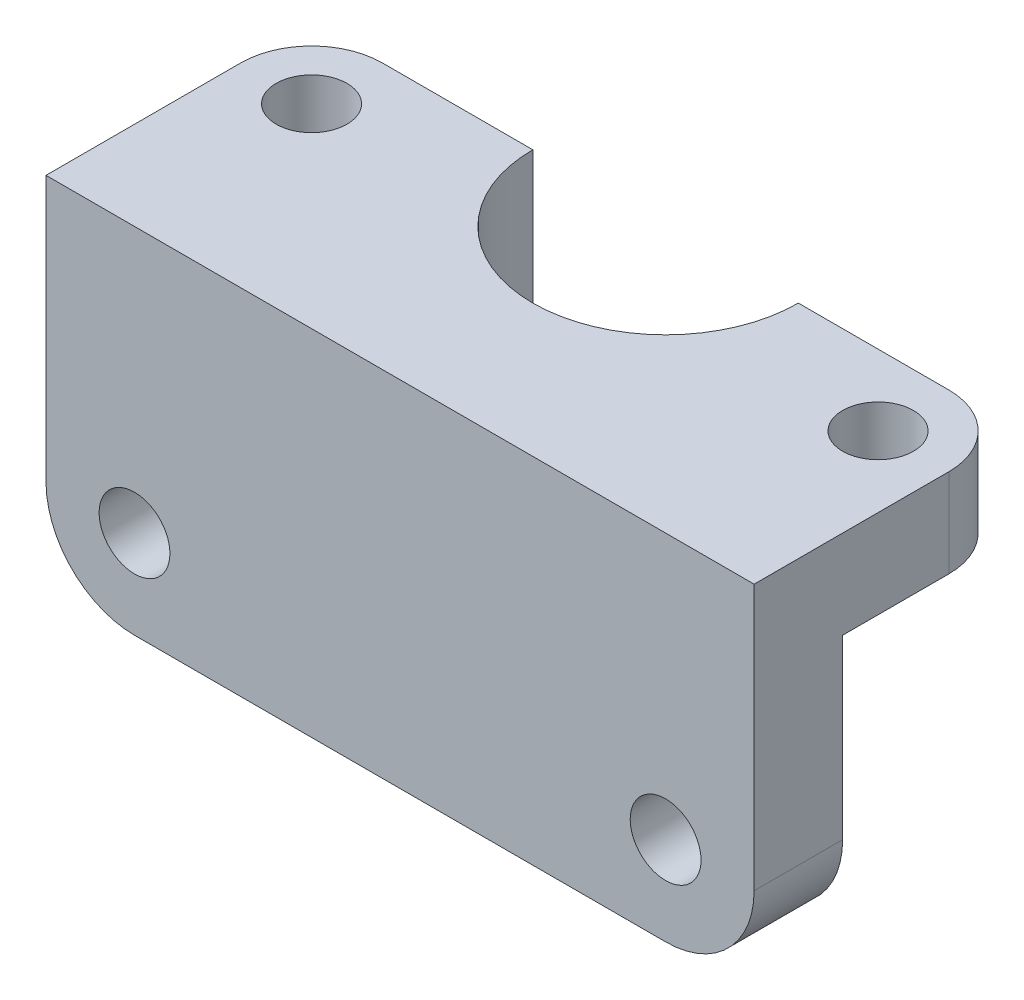
ISO-10303-21;
HEADER;
FILE_DESCRIPTION(('STEP AP214'),'2;1');
FILE_NAME('part.step','',(''),(''),'','','');
FILE_SCHEMA(('AUTOMOTIVE_DESIGN { 1 0 10303 214 1 1 1 1 }'));
ENDSEC;
DATA;
#1=APPLICATION_CONTEXT('core data for automotive mechanical design processes');
#2=APPLICATION_PROTOCOL_DEFINITION('international standard','automotive_design',2000,#1);
#3=PRODUCT_CONTEXT('',#1,'mechanical');
#4=PRODUCT('Part','Part','',(#3));
#5=PRODUCT_RELATED_PRODUCT_CATEGORY('part','',(#4));
#6=PRODUCT_DEFINITION_FORMATION('','',#4);
#7=PRODUCT_DEFINITION_CONTEXT('part definition',#1,'design');
#8=PRODUCT_DEFINITION('design','',#6,#7);
#9=PRODUCT_DEFINITION_SHAPE('','',#8);
#10=(LENGTH_UNIT() NAMED_UNIT(*) SI_UNIT(.MILLI.,.METRE.));
#11=(NAMED_UNIT(*) PLANE_ANGLE_UNIT() SI_UNIT($,.RADIAN.));
#12=(NAMED_UNIT(*) SI_UNIT($,.STERADIAN.) SOLID_ANGLE_UNIT());
#13=UNCERTAINTY_MEASURE_WITH_UNIT(LENGTH_MEASURE(1.E-05),#10,'distance_accuracy_value','');
#14=(GEOMETRIC_REPRESENTATION_CONTEXT(3) GLOBAL_UNCERTAINTY_ASSIGNED_CONTEXT((#13)) GLOBAL_UNIT_ASSIGNED_CONTEXT((#10,
#11,#12)) REPRESENTATION_CONTEXT('',''));
#15=CARTESIAN_POINT('',(0.,0.,0.));
#16=DIRECTION('',(0.,0.,1.));
#17=DIRECTION('',(1.,0.,0.));
#18=AXIS2_PLACEMENT_3D('',#15,#16,#17);
#19=CARTESIAN_POINT('',(8.00000000000006,-10.,-20.));
#20=DIRECTION('',(0.,0.,-1.));
#21=DIRECTION('',(-1.,0.,0.));
#22=AXIS2_PLACEMENT_3D('',#19,#20,#21);
#23=PLANE('',#22);
#24=DIRECTION('',(0.,-1.,0.));
#25=VECTOR('',#24,1.);
#26=CARTESIAN_POINT('',(55.,0.,-20.));
#27=LINE('',#26,#25);
#28=CARTESIAN_POINT('',(55.,0.,-20.));
#29=VERTEX_POINT('',#28);
#30=CARTESIAN_POINT('',(55.,-35.,-20.));
#31=VERTEX_POINT('',#30);
#32=EDGE_CURVE('E62',#29,#31,#27,.T.);
#33=ORIENTED_EDGE('',*,*,#32,.F.);
#34=DIRECTION('',(-1.,0.,0.));
#35=VECTOR('',#34,1.);
#36=CARTESIAN_POINT('',(8.00000000000006,0.,-20.));
#37=LINE('',#36,#35);
#38=CARTESIAN_POINT('',(71.9999999999999,0.,-20.));
#39=VERTEX_POINT('',#38);
#40=EDGE_CURVE('E179',#39,#29,#37,.T.);
#41=ORIENTED_EDGE('',*,*,#40,.F.);
#42=DIRECTION('',(0.,1.,0.));
#43=VECTOR('',#42,1.);
#44=CARTESIAN_POINT('',(71.9999999999999,-10.,-20.));
#45=LINE('',#44,#43);
#46=CARTESIAN_POINT('',(71.9999999999999,-10.,-20.));
#47=VERTEX_POINT('',#46);
#48=EDGE_CURVE('E199',#47,#39,#45,.T.);
#49=ORIENTED_EDGE('',*,*,#48,.F.);
#50=DIRECTION('',(-1.,0.,0.));
#51=VECTOR('',#50,1.);
#52=CARTESIAN_POINT('',(8.00000000000006,-10.,-20.));
#53=LINE('',#52,#51);
#54=CARTESIAN_POINT('',(60.,-10.,-20.));
#55=VERTEX_POINT('',#54);
#56=EDGE_CURVE('E295',#47,#55,#53,.T.);
#57=ORIENTED_EDGE('',*,*,#56,.T.);
#58=DIRECTION('',(0.,1.,0.));
#59=VECTOR('',#58,1.);
#60=CARTESIAN_POINT('',(60.,-35.,-20.));
#61=LINE('',#60,#59);
#62=CARTESIAN_POINT('',(60.,-35.,-20.));
#63=VERTEX_POINT('',#62);
#64=EDGE_CURVE('E281',#63,#55,#61,.T.);
#65=ORIENTED_EDGE('',*,*,#64,.F.);
#66=DIRECTION('',(1.,0.,0.));
#67=VECTOR('',#66,1.);
#68=CARTESIAN_POINT('',(20.,-35.,-20.));
#69=LINE('',#68,#67);
#70=EDGE_CURVE('E269',#31,#63,#69,.T.);
#71=ORIENTED_EDGE('',*,*,#70,.F.);
#72=EDGE_LOOP('',(#33,#41,#49,#57,#65,#71));
#73=FACE_BOUND('',#72,.T.);
#74=ADVANCED_FACE('F44',(#73),#23,.T.);
#75=CARTESIAN_POINT('',(70.,-30.,0.));
#76=DIRECTION('',(0.,0.,1.));
#77=DIRECTION('',(1.,0.,0.));
#78=AXIS2_PLACEMENT_3D('',#75,#76,#77);
#79=PLANE('',#78);
#80=CARTESIAN_POINT('',(70.,-30.,0.));
#81=DIRECTION('',(0.,0.,-1.));
#82=DIRECTION('',(-1.,0.,0.));
#83=AXIS2_PLACEMENT_3D('',#80,#81,#82);
#84=CIRCLE('',#83,4.00000000000001);
#85=CARTESIAN_POINT('',(66.,-30.,0.));
#86=VERTEX_POINT('',#85);
#87=EDGE_CURVE('E242',#86,#86,#84,.T.);
#88=ORIENTED_EDGE('',*,*,#87,.F.);
#89=EDGE_LOOP('',(#88));
#90=FACE_BOUND('',#89,.T.);
#91=CARTESIAN_POINT('',(10.,-30.,0.));
#92=DIRECTION('',(0.,0.,-1.));
#93=DIRECTION('',(-1.,0.,0.));
#94=AXIS2_PLACEMENT_3D('',#91,#92,#93);
#95=CIRCLE('',#94,4.);
#96=CARTESIAN_POINT('',(6.,-30.,0.));
#97=VERTEX_POINT('',#96);
#98=EDGE_CURVE('E246',#97,#97,#95,.T.);
#99=ORIENTED_EDGE('',*,*,#98,.F.);
#100=EDGE_LOOP('',(#99));
#101=FACE_BOUND('',#100,.T.);
#102=DIRECTION('',(0.,1.,0.));
#103=VECTOR('',#102,1.);
#104=CARTESIAN_POINT('',(20.,-35.,0.));
#105=LINE('',#104,#103);
#106=CARTESIAN_POINT('',(20.,-35.,0.));
#107=VERTEX_POINT('',#106);
#108=CARTESIAN_POINT('',(20.,-10.,0.));
#109=VERTEX_POINT('',#108);
#110=EDGE_CURVE('E186',#107,#109,#105,.T.);
#111=ORIENTED_EDGE('',*,*,#110,.F.);
#112=DIRECTION('',(-1.,0.,0.));
#113=VECTOR('',#112,1.);
#114=CARTESIAN_POINT('',(40.,-35.,0.));
#115=LINE('',#114,#113);
#116=CARTESIAN_POINT('',(60.,-35.,0.));
#117=VERTEX_POINT('',#116);
#118=EDGE_CURVE('E66',#117,#107,#115,.T.);
#119=ORIENTED_EDGE('',*,*,#118,.F.);
#120=DIRECTION('',(0.,1.,0.));
#121=VECTOR('',#120,1.);
#122=CARTESIAN_POINT('',(60.,-35.,0.));
#123=LINE('',#122,#121);
#124=CARTESIAN_POINT('',(60.,-10.,0.));
#125=VERTEX_POINT('',#124);
#126=EDGE_CURVE('E274',#117,#125,#123,.T.);
#127=ORIENTED_EDGE('',*,*,#126,.T.);
#128=DIRECTION('',(1.,0.,0.));
#129=VECTOR('',#128,1.);
#130=CARTESIAN_POINT('',(80.,-10.,0.));
#131=LINE('',#130,#129);
#132=CARTESIAN_POINT('',(80.,-10.,0.));
#133=VERTEX_POINT('',#132);
#134=EDGE_CURVE('E303',#125,#133,#131,.T.);
#135=ORIENTED_EDGE('',*,*,#134,.T.);
#136=DIRECTION('',(0.,1.,0.));
#137=VECTOR('',#136,1.);
#138=CARTESIAN_POINT('',(80.,0.,0.));
#139=LINE('',#138,#137);
#140=CARTESIAN_POINT('',(80.,-29.9999999999999,0.));
#141=VERTEX_POINT('',#140);
#142=EDGE_CURVE('E210',#141,#133,#139,.T.);
#143=ORIENTED_EDGE('',*,*,#142,.F.);
#144=CARTESIAN_POINT('',(70.,-30.,0.));
#145=DIRECTION('',(0.,0.,1.));
#146=DIRECTION('',(1.,0.,0.));
#147=AXIS2_PLACEMENT_3D('',#144,#145,#146);
#148=CIRCLE('',#147,10.);
#149=CARTESIAN_POINT('',(69.9999999999999,-40.,0.));
#150=VERTEX_POINT('',#149);
#151=EDGE_CURVE('E224',#150,#141,#148,.T.);
#152=ORIENTED_EDGE('',*,*,#151,.F.);
#153=DIRECTION('',(1.,0.,0.));
#154=VECTOR('',#153,1.);
#155=CARTESIAN_POINT('',(69.9999999999999,-40.,0.));
#156=LINE('',#155,#154);
#157=CARTESIAN_POINT('',(10.0000000000001,-40.,0.));
#158=VERTEX_POINT('',#157);
#159=EDGE_CURVE('E222',#158,#150,#156,.T.);
#160=ORIENTED_EDGE('',*,*,#159,.F.);
#161=CARTESIAN_POINT('',(10.,-30.,0.));
#162=DIRECTION('',(0.,0.,1.));
#163=DIRECTION('',(-1.,0.,0.));
#164=AXIS2_PLACEMENT_3D('',#161,#162,#163);
#165=CIRCLE('',#164,10.);
#166=CARTESIAN_POINT('',(0.,-30.,0.));
#167=VERTEX_POINT('',#166);
#168=EDGE_CURVE('E218',#167,#158,#165,.T.);
#169=ORIENTED_EDGE('',*,*,#168,.F.);
#170=DIRECTION('',(0.,-1.,0.));
#171=VECTOR('',#170,1.);
#172=CARTESIAN_POINT('',(0.,-29.9999999999999,0.));
#173=LINE('',#172,#171);
#174=CARTESIAN_POINT('',(0.,-10.,0.));
#175=VERTEX_POINT('',#174);
#176=EDGE_CURVE('E191',#175,#167,#173,.T.);
#177=ORIENTED_EDGE('',*,*,#176,.F.);
#178=EDGE_CURVE('E304',#175,#109,#131,.T.);
#179=ORIENTED_EDGE('',*,*,#178,.T.);
#180=EDGE_LOOP('',(#111,#119,#127,#135,#143,#152,#160,#169,#177,#179));
#181=FACE_BOUND('',#180,.T.);
#182=ADVANCED_FACE('F329',(#90,#101,#181),#79,.F.);
#183=CARTESIAN_POINT('',(72.,-10.,-12.));
#184=DIRECTION('',(0.,1.,0.));
#185=DIRECTION('',(0.,0.,1.));
#186=AXIS2_PLACEMENT_3D('',#183,#184,#185);
#187=PLANE('',#186);
#188=CARTESIAN_POINT('',(8.,-10.,-12.));
#189=DIRECTION('',(0.,-1.,0.));
#190=DIRECTION('',(0.,0.,-1.));
#191=AXIS2_PLACEMENT_3D('',#188,#189,#190);
#192=CIRCLE('',#191,4.);
#193=CARTESIAN_POINT('',(8.,-10.,-16.));
#194=VERTEX_POINT('',#193);
#195=EDGE_CURVE('E252',#194,#194,#192,.T.);
#196=ORIENTED_EDGE('',*,*,#195,.F.);
#197=EDGE_LOOP('',(#196));
#198=FACE_BOUND('',#197,.T.);
#199=DIRECTION('',(0.,0.,-1.));
#200=VECTOR('',#199,1.);
#201=CARTESIAN_POINT('',(20.,-10.,0.));
#202=LINE('',#201,#200);
#203=CARTESIAN_POINT('',(20.,-10.,-20.));
#204=VERTEX_POINT('',#203);
#205=EDGE_CURVE('E262',#109,#204,#202,.T.);
#206=ORIENTED_EDGE('',*,*,#205,.F.);
#207=ORIENTED_EDGE('',*,*,#178,.F.);
#208=DIRECTION('',(0.,0.,1.));
#209=VECTOR('',#208,1.);
#210=CARTESIAN_POINT('',(0.,-10.,0.));
#211=LINE('',#210,#209);
#212=CARTESIAN_POINT('',(0.,-10.,-11.9999999999999));
#213=VERTEX_POINT('',#212);
#214=EDGE_CURVE('E299',#213,#175,#211,.T.);
#215=ORIENTED_EDGE('',*,*,#214,.F.);
#216=CARTESIAN_POINT('',(8.,-10.,-12.));
#217=DIRECTION('',(0.,1.,0.));
#218=DIRECTION('',(0.,0.,1.));
#219=AXIS2_PLACEMENT_3D('',#216,#217,#218);
#220=CIRCLE('',#219,8.);
#221=CARTESIAN_POINT('',(8.00000000000006,-10.,-20.));
#222=VERTEX_POINT('',#221);
#223=EDGE_CURVE('E293',#222,#213,#220,.T.);
#224=ORIENTED_EDGE('',*,*,#223,.F.);
#225=EDGE_CURVE('E292',#204,#222,#53,.T.);
#226=ORIENTED_EDGE('',*,*,#225,.F.);
#227=EDGE_LOOP('',(#206,#207,#215,#224,#226));
#228=FACE_BOUND('',#227,.T.);
#229=ADVANCED_FACE('F347',(#198,#228),#187,.F.);
#230=CARTESIAN_POINT('',(72.,-10.,-12.));
#231=DIRECTION('',(0.,-1.,0.));
#232=DIRECTION('',(0.,0.,-1.));
#233=AXIS2_PLACEMENT_3D('',#230,#231,#232);
#234=CIRCLE('',#233,4.00000000000001);
#235=CARTESIAN_POINT('',(72.,-10.,-16.));
#236=VERTEX_POINT('',#235);
#237=EDGE_CURVE('E248',#236,#236,#234,.T.);
#238=ORIENTED_EDGE('',*,*,#237,.F.);
#239=EDGE_LOOP('',(#238));
#240=FACE_BOUND('',#239,.T.);
#241=DIRECTION('',(0.,0.,1.));
#242=VECTOR('',#241,1.);
#243=CARTESIAN_POINT('',(60.,-10.,-20.));
#244=LINE('',#243,#242);
#245=EDGE_CURVE('E268',#55,#125,#244,.T.);
#246=ORIENTED_EDGE('',*,*,#245,.F.);
#247=ORIENTED_EDGE('',*,*,#56,.F.);
#248=CARTESIAN_POINT('',(72.,-10.,-12.));
#249=DIRECTION('',(0.,1.,0.));
#250=DIRECTION('',(0.,0.,1.));
#251=AXIS2_PLACEMENT_3D('',#248,#249,#250);
#252=CIRCLE('',#251,8.);
#253=CARTESIAN_POINT('',(80.,-10.,-11.9999999999999));
#254=VERTEX_POINT('',#253);
#255=EDGE_CURVE('E193',#254,#47,#252,.T.);
#256=ORIENTED_EDGE('',*,*,#255,.F.);
#257=DIRECTION('',(0.,0.,-1.));
#258=VECTOR('',#257,1.);
#259=CARTESIAN_POINT('',(80.,-10.,-11.9999999999999));
#260=LINE('',#259,#258);
#261=EDGE_CURVE('E205',#133,#254,#260,.T.);
#262=ORIENTED_EDGE('',*,*,#261,.F.);
#263=ORIENTED_EDGE('',*,*,#134,.F.);
#264=EDGE_LOOP('',(#246,#247,#256,#262,#263));
#265=FACE_BOUND('',#264,.T.);
#266=ADVANCED_FACE('F311',(#240,#265),#187,.F.);
#267=CARTESIAN_POINT('',(0.,-29.9999999999999,10.));
#268=DIRECTION('',(1.,0.,0.));
#269=DIRECTION('',(0.,0.,-1.));
#270=AXIS2_PLACEMENT_3D('',#267,#268,#269);
#271=PLANE('',#270);
#272=DIRECTION('',(0.,0.,-1.));
#273=VECTOR('',#272,1.);
#274=CARTESIAN_POINT('',(0.,0.,10.));
#275=LINE('',#274,#273);
#276=CARTESIAN_POINT('',(0.,0.,10.));
#277=VERTEX_POINT('',#276);
#278=CARTESIAN_POINT('',(0.,0.,-11.9999999999999));
#279=VERTEX_POINT('',#278);
#280=EDGE_CURVE('E220',#277,#279,#275,.T.);
#281=ORIENTED_EDGE('',*,*,#280,.T.);
#282=DIRECTION('',(0.,1.,0.));
#283=VECTOR('',#282,1.);
#284=CARTESIAN_POINT('',(0.,-10.,-11.9999999999999));
#285=LINE('',#284,#283);
#286=EDGE_CURVE('E198',#213,#279,#285,.T.);
#287=ORIENTED_EDGE('',*,*,#286,.F.);
#288=ORIENTED_EDGE('',*,*,#214,.T.);
#289=ORIENTED_EDGE('',*,*,#176,.T.);
#290=DIRECTION('',(0.,0.,-1.));
#291=VECTOR('',#290,1.);
#292=CARTESIAN_POINT('',(0.,-30.,10.));
#293=LINE('',#292,#291);
#294=CARTESIAN_POINT('',(0.,-30.,10.));
#295=VERTEX_POINT('',#294);
#296=EDGE_CURVE('E11',#295,#167,#293,.T.);
#297=ORIENTED_EDGE('',*,*,#296,.F.);
#298=DIRECTION('',(0.,-1.,0.));
#299=VECTOR('',#298,1.);
#300=CARTESIAN_POINT('',(0.,-29.9999999999999,10.));
#301=LINE('',#300,#299);
#302=EDGE_CURVE('E201',#277,#295,#301,.T.);
#303=ORIENTED_EDGE('',*,*,#302,.F.);
#304=EDGE_LOOP('',(#281,#287,#288,#289,#297,#303));
#305=FACE_BOUND('',#304,.T.);
#306=ADVANCED_FACE('F50',(#305),#271,.F.);
#307=CARTESIAN_POINT('',(10.,-30.,10.));
#308=DIRECTION('',(0.,0.,-1.));
#309=DIRECTION('',(-1.,0.,0.));
#310=AXIS2_PLACEMENT_3D('',#307,#308,#309);
#311=CYLINDRICAL_SURFACE('',#310,10.);
#312=ORIENTED_EDGE('',*,*,#168,.T.);
#313=DIRECTION('',(0.,0.,-1.));
#314=VECTOR('',#313,1.);
#315=CARTESIAN_POINT('',(10.0000000000001,-40.,10.));
#316=LINE('',#315,#314);
#317=CARTESIAN_POINT('',(10.0000000000001,-40.,10.));
#318=VERTEX_POINT('',#317);
#319=EDGE_CURVE('E53',#318,#158,#316,.T.);
#320=ORIENTED_EDGE('',*,*,#319,.F.);
#321=CARTESIAN_POINT('',(10.,-30.,10.));
#322=DIRECTION('',(0.,0.,1.));
#323=DIRECTION('',(-1.,0.,0.));
#324=AXIS2_PLACEMENT_3D('',#321,#322,#323);
#325=CIRCLE('',#324,10.);
#326=EDGE_CURVE('E206',#295,#318,#325,.T.);
#327=ORIENTED_EDGE('',*,*,#326,.F.);
#328=ORIENTED_EDGE('',*,*,#296,.T.);
#329=EDGE_LOOP('',(#312,#320,#327,#328));
#330=FACE_BOUND('',#329,.T.);
#331=ADVANCED_FACE('F359',(#330),#311,.T.);
#332=CARTESIAN_POINT('',(69.9999999999999,-40.,10.));
#333=DIRECTION('',(0.,1.,0.));
#334=DIRECTION('',(0.,0.,1.));
#335=AXIS2_PLACEMENT_3D('',#332,#333,#334);
#336=PLANE('',#335);
#337=ORIENTED_EDGE('',*,*,#159,.T.);
#338=DIRECTION('',(0.,0.,-1.));
#339=VECTOR('',#338,1.);
#340=CARTESIAN_POINT('',(69.9999999999999,-40.,10.));
#341=LINE('',#340,#339);
#342=CARTESIAN_POINT('',(69.9999999999999,-40.,10.));
#343=VERTEX_POINT('',#342);
#344=EDGE_CURVE('E232',#343,#150,#341,.T.);
#345=ORIENTED_EDGE('',*,*,#344,.F.);
#346=DIRECTION('',(1.,0.,0.));
#347=VECTOR('',#346,1.);
#348=CARTESIAN_POINT('',(69.9999999999999,-40.,10.));
#349=LINE('',#348,#347);
#350=EDGE_CURVE('E207',#318,#343,#349,.T.);
#351=ORIENTED_EDGE('',*,*,#350,.F.);
#352=ORIENTED_EDGE('',*,*,#319,.T.);
#353=EDGE_LOOP('',(#337,#345,#351,#352));
#354=FACE_BOUND('',#353,.T.);
#355=ADVANCED_FACE('F360',(#354),#336,.F.);
#356=CARTESIAN_POINT('',(70.,-30.,10.));
#357=DIRECTION('',(0.,0.,-1.));
#358=DIRECTION('',(-1.,0.,0.));
#359=AXIS2_PLACEMENT_3D('',#356,#357,#358);
#360=CYLINDRICAL_SURFACE('',#359,10.);
#361=ORIENTED_EDGE('',*,*,#151,.T.);
#362=DIRECTION('',(0.,0.,-1.));
#363=VECTOR('',#362,1.);
#364=CARTESIAN_POINT('',(80.,-29.9999999999999,10.));
#365=LINE('',#364,#363);
#366=CARTESIAN_POINT('',(80.,-29.9999999999999,10.));
#367=VERTEX_POINT('',#366);
#368=EDGE_CURVE('E230',#367,#141,#365,.T.);
#369=ORIENTED_EDGE('',*,*,#368,.F.);
#370=CARTESIAN_POINT('',(70.,-30.,10.));
#371=DIRECTION('',(0.,0.,1.));
#372=DIRECTION('',(1.,0.,0.));
#373=AXIS2_PLACEMENT_3D('',#370,#371,#372);
#374=CIRCLE('',#373,10.);
#375=EDGE_CURVE('E211',#343,#367,#374,.T.);
#376=ORIENTED_EDGE('',*,*,#375,.F.);
#377=ORIENTED_EDGE('',*,*,#344,.T.);
#378=EDGE_LOOP('',(#361,#369,#376,#377));
#379=FACE_BOUND('',#378,.T.);
#380=ADVANCED_FACE('F330',(#379),#360,.T.);
#381=CARTESIAN_POINT('',(80.,0.,10.));
#382=DIRECTION('',(-1.,0.,0.));
#383=DIRECTION('',(0.,0.,1.));
#384=AXIS2_PLACEMENT_3D('',#381,#382,#383);
#385=PLANE('',#384);
#386=ORIENTED_EDGE('',*,*,#142,.T.);
#387=ORIENTED_EDGE('',*,*,#261,.T.);
#388=DIRECTION('',(0.,1.,0.));
#389=VECTOR('',#388,1.);
#390=CARTESIAN_POINT('',(80.,-10.,-11.9999999999999));
#391=LINE('',#390,#389);
#392=CARTESIAN_POINT('',(80.,0.,-11.9999999999999));
#393=VERTEX_POINT('',#392);
#394=EDGE_CURVE('E194',#254,#393,#391,.T.);
#395=ORIENTED_EDGE('',*,*,#394,.T.);
#396=DIRECTION('',(0.,0.,-1.));
#397=VECTOR('',#396,1.);
#398=CARTESIAN_POINT('',(80.,0.,10.));
#399=LINE('',#398,#397);
#400=CARTESIAN_POINT('',(80.,0.,10.));
#401=VERTEX_POINT('',#400);
#402=EDGE_CURVE('E229',#401,#393,#399,.T.);
#403=ORIENTED_EDGE('',*,*,#402,.F.);
#404=DIRECTION('',(0.,1.,0.));
#405=VECTOR('',#404,1.);
#406=CARTESIAN_POINT('',(80.,0.,10.));
#407=LINE('',#406,#405);
#408=EDGE_CURVE('E213',#367,#401,#407,.T.);
#409=ORIENTED_EDGE('',*,*,#408,.F.);
#410=ORIENTED_EDGE('',*,*,#368,.T.);
#411=EDGE_LOOP('',(#386,#387,#395,#403,#409,#410));
#412=FACE_BOUND('',#411,.T.);
#413=ADVANCED_FACE('F307',(#412),#385,.F.);
#414=CARTESIAN_POINT('',(0.,0.,10.));
#415=DIRECTION('',(0.,-1.,0.));
#416=DIRECTION('',(0.,0.,-1.));
#417=AXIS2_PLACEMENT_3D('',#414,#415,#416);
#418=PLANE('',#417);
#419=CARTESIAN_POINT('',(72.,0.,-12.));
#420=DIRECTION('',(0.,-1.,0.));
#421=DIRECTION('',(0.,0.,-1.));
#422=AXIS2_PLACEMENT_3D('',#419,#420,#421);
#423=CIRCLE('',#422,4.00000000000001);
#424=CARTESIAN_POINT('',(72.,0.,-16.));
#425=VERTEX_POINT('',#424);
#426=EDGE_CURVE('E47',#425,#425,#423,.T.);
#427=ORIENTED_EDGE('',*,*,#426,.T.);
#428=EDGE_LOOP('',(#427));
#429=FACE_BOUND('',#428,.T.);
#430=CARTESIAN_POINT('',(8.,0.,-12.));
#431=DIRECTION('',(0.,-1.,0.));
#432=DIRECTION('',(0.,0.,-1.));
#433=AXIS2_PLACEMENT_3D('',#430,#431,#432);
#434=CIRCLE('',#433,4.);
#435=CARTESIAN_POINT('',(8.,0.,-16.));
#436=VERTEX_POINT('',#435);
#437=EDGE_CURVE('E243',#436,#436,#434,.T.);
#438=ORIENTED_EDGE('',*,*,#437,.T.);
#439=EDGE_LOOP('',(#438));
#440=FACE_BOUND('',#439,.T.);
#441=ORIENTED_EDGE('',*,*,#40,.T.);
#442=CARTESIAN_POINT('',(40.,0.,-20.));
#443=DIRECTION('',(0.,-1.,0.));
#444=DIRECTION('',(0.,0.,-1.));
#445=AXIS2_PLACEMENT_3D('',#442,#443,#444);
#446=CIRCLE('',#445,15.);
#447=CARTESIAN_POINT('',(25.,0.,-20.));
#448=VERTEX_POINT('',#447);
#449=EDGE_CURVE('E165',#29,#448,#446,.T.);
#450=ORIENTED_EDGE('',*,*,#449,.T.);
#451=CARTESIAN_POINT('',(8.00000000000006,0.,-20.));
#452=VERTEX_POINT('',#451);
#453=EDGE_CURVE('E174',#448,#452,#37,.T.);
#454=ORIENTED_EDGE('',*,*,#453,.T.);
#455=CARTESIAN_POINT('',(8.,0.,-12.));
#456=DIRECTION('',(0.,1.,0.));
#457=DIRECTION('',(0.,0.,1.));
#458=AXIS2_PLACEMENT_3D('',#455,#456,#457);
#459=CIRCLE('',#458,8.);
#460=EDGE_CURVE('E183',#452,#279,#459,.T.);
#461=ORIENTED_EDGE('',*,*,#460,.T.);
#462=ORIENTED_EDGE('',*,*,#280,.F.);
#463=DIRECTION('',(-1.,0.,0.));
#464=VECTOR('',#463,1.);
#465=CARTESIAN_POINT('',(0.,0.,10.));
#466=LINE('',#465,#464);
#467=EDGE_CURVE('E214',#401,#277,#466,.T.);
#468=ORIENTED_EDGE('',*,*,#467,.F.);
#469=ORIENTED_EDGE('',*,*,#402,.T.);
#470=CARTESIAN_POINT('',(72.,0.,-12.));
#471=DIRECTION('',(0.,1.,0.));
#472=DIRECTION('',(0.,0.,1.));
#473=AXIS2_PLACEMENT_3D('',#470,#471,#472);
#474=CIRCLE('',#473,8.);
#475=EDGE_CURVE('E181',#393,#39,#474,.T.);
#476=ORIENTED_EDGE('',*,*,#475,.T.);
#477=EDGE_LOOP('',(#441,#450,#454,#461,#462,#468,#469,#476));
#478=FACE_BOUND('',#477,.T.);
#479=ADVANCED_FACE('F171',(#429,#440,#478),#418,.F.);
#480=CARTESIAN_POINT('',(70.,-30.,10.));
#481=DIRECTION('',(0.,0.,1.));
#482=DIRECTION('',(1.,0.,0.));
#483=AXIS2_PLACEMENT_3D('',#480,#481,#482);
#484=PLANE('',#483);
#485=CARTESIAN_POINT('',(70.,-30.,10.));
#486=DIRECTION('',(0.,0.,1.));
#487=DIRECTION('',(1.,0.,0.));
#488=AXIS2_PLACEMENT_3D('',#485,#486,#487);
#489=CIRCLE('',#488,4.00000000000001);
#490=CARTESIAN_POINT('',(74.,-30.,10.));
#491=VERTEX_POINT('',#490);
#492=EDGE_CURVE('E241',#491,#491,#489,.T.);
#493=ORIENTED_EDGE('',*,*,#492,.F.);
#494=EDGE_LOOP('',(#493));
#495=FACE_BOUND('',#494,.T.);
#496=CARTESIAN_POINT('',(10.,-30.,10.));
#497=DIRECTION('',(0.,0.,1.));
#498=DIRECTION('',(1.,0.,0.));
#499=AXIS2_PLACEMENT_3D('',#496,#497,#498);
#500=CIRCLE('',#499,4.);
#501=CARTESIAN_POINT('',(14.,-30.,10.));
#502=VERTEX_POINT('',#501);
#503=EDGE_CURVE('E236',#502,#502,#500,.T.);
#504=ORIENTED_EDGE('',*,*,#503,.F.);
#505=EDGE_LOOP('',(#504));
#506=FACE_BOUND('',#505,.T.);
#507=ORIENTED_EDGE('',*,*,#302,.T.);
#508=ORIENTED_EDGE('',*,*,#326,.T.);
#509=ORIENTED_EDGE('',*,*,#350,.T.);
#510=ORIENTED_EDGE('',*,*,#375,.T.);
#511=ORIENTED_EDGE('',*,*,#408,.T.);
#512=ORIENTED_EDGE('',*,*,#467,.T.);
#513=EDGE_LOOP('',(#507,#508,#509,#510,#511,#512));
#514=FACE_BOUND('',#513,.T.);
#515=ADVANCED_FACE('F325',(#495,#506,#514),#484,.T.);
#516=CARTESIAN_POINT('',(72.,-10.,-12.));
#517=DIRECTION('',(0.,1.,0.));
#518=DIRECTION('',(0.,0.,1.));
#519=AXIS2_PLACEMENT_3D('',#516,#517,#518);
#520=CYLINDRICAL_SURFACE('',#519,8.);
#521=ORIENTED_EDGE('',*,*,#475,.F.);
#522=ORIENTED_EDGE('',*,*,#394,.F.);
#523=ORIENTED_EDGE('',*,*,#255,.T.);
#524=ORIENTED_EDGE('',*,*,#48,.T.);
#525=EDGE_LOOP('',(#521,#522,#523,#524));
#526=FACE_BOUND('',#525,.T.);
#527=ADVANCED_FACE('F316',(#526),#520,.T.);
#528=CARTESIAN_POINT('',(8.,-10.,-12.));
#529=DIRECTION('',(0.,1.,0.));
#530=DIRECTION('',(0.,0.,1.));
#531=AXIS2_PLACEMENT_3D('',#528,#529,#530);
#532=CYLINDRICAL_SURFACE('',#531,8.);
#533=ORIENTED_EDGE('',*,*,#460,.F.);
#534=DIRECTION('',(0.,1.,0.));
#535=VECTOR('',#534,1.);
#536=CARTESIAN_POINT('',(8.00000000000006,-10.,-20.));
#537=LINE('',#536,#535);
#538=EDGE_CURVE('E182',#222,#452,#537,.T.);
#539=ORIENTED_EDGE('',*,*,#538,.F.);
#540=ORIENTED_EDGE('',*,*,#223,.T.);
#541=ORIENTED_EDGE('',*,*,#286,.T.);
#542=EDGE_LOOP('',(#533,#539,#540,#541));
#543=FACE_BOUND('',#542,.T.);
#544=ADVANCED_FACE('F353',(#543),#532,.T.);
#545=DIRECTION('',(0.,-1.,0.));
#546=VECTOR('',#545,1.);
#547=CARTESIAN_POINT('',(25.,0.,-20.));
#548=LINE('',#547,#546);
#549=CARTESIAN_POINT('',(25.,-35.,-20.));
#550=VERTEX_POINT('',#549);
#551=EDGE_CURVE('E157',#448,#550,#548,.T.);
#552=ORIENTED_EDGE('',*,*,#551,.T.);
#553=CARTESIAN_POINT('',(20.,-35.,-20.));
#554=VERTEX_POINT('',#553);
#555=EDGE_CURVE('E271',#554,#550,#69,.T.);
#556=ORIENTED_EDGE('',*,*,#555,.F.);
#557=DIRECTION('',(0.,1.,0.));
#558=VECTOR('',#557,1.);
#559=CARTESIAN_POINT('',(20.,-35.,-20.));
#560=LINE('',#559,#558);
#561=EDGE_CURVE('E283',#554,#204,#560,.T.);
#562=ORIENTED_EDGE('',*,*,#561,.T.);
#563=ORIENTED_EDGE('',*,*,#225,.T.);
#564=ORIENTED_EDGE('',*,*,#538,.T.);
#565=ORIENTED_EDGE('',*,*,#453,.F.);
#566=EDGE_LOOP('',(#552,#556,#562,#563,#564,#565));
#567=FACE_BOUND('',#566,.T.);
#568=ADVANCED_FACE('F180',(#567),#23,.T.);
#569=CARTESIAN_POINT('',(20.,-35.,0.));
#570=DIRECTION('',(1.,0.,0.));
#571=DIRECTION('',(0.,0.,-1.));
#572=AXIS2_PLACEMENT_3D('',#569,#570,#571);
#573=PLANE('',#572);
#574=ORIENTED_EDGE('',*,*,#205,.T.);
#575=ORIENTED_EDGE('',*,*,#561,.F.);
#576=DIRECTION('',(0.,0.,-1.));
#577=VECTOR('',#576,1.);
#578=CARTESIAN_POINT('',(20.,-35.,0.));
#579=LINE('',#578,#577);
#580=EDGE_CURVE('E270',#107,#554,#579,.T.);
#581=ORIENTED_EDGE('',*,*,#580,.F.);
#582=ORIENTED_EDGE('',*,*,#110,.T.);
#583=EDGE_LOOP('',(#574,#575,#581,#582));
#584=FACE_BOUND('',#583,.T.);
#585=ADVANCED_FACE('F345',(#584),#573,.F.);
#586=CARTESIAN_POINT('',(60.,-35.,-20.));
#587=DIRECTION('',(-1.,0.,0.));
#588=DIRECTION('',(0.,0.,1.));
#589=AXIS2_PLACEMENT_3D('',#586,#587,#588);
#590=PLANE('',#589);
#591=ORIENTED_EDGE('',*,*,#245,.T.);
#592=ORIENTED_EDGE('',*,*,#126,.F.);
#593=DIRECTION('',(0.,0.,1.));
#594=VECTOR('',#593,1.);
#595=CARTESIAN_POINT('',(60.,-35.,-20.));
#596=LINE('',#595,#594);
#597=EDGE_CURVE('E272',#63,#117,#596,.T.);
#598=ORIENTED_EDGE('',*,*,#597,.F.);
#599=ORIENTED_EDGE('',*,*,#64,.T.);
#600=EDGE_LOOP('',(#591,#592,#598,#599));
#601=FACE_BOUND('',#600,.T.);
#602=ADVANCED_FACE('F333',(#601),#590,.F.);
#603=CARTESIAN_POINT('',(0.,-35.,0.));
#604=DIRECTION('',(0.,-1.,0.));
#605=DIRECTION('',(0.,0.,-1.));
#606=AXIS2_PLACEMENT_3D('',#603,#604,#605);
#607=PLANE('',#606);
#608=CARTESIAN_POINT('',(40.,-35.,-20.));
#609=DIRECTION('',(0.,-1.,0.));
#610=DIRECTION('',(0.,0.,-1.));
#611=AXIS2_PLACEMENT_3D('',#608,#609,#610);
#612=CIRCLE('',#611,15.);
#613=EDGE_CURVE('E162',#31,#550,#612,.T.);
#614=ORIENTED_EDGE('',*,*,#613,.F.);
#615=ORIENTED_EDGE('',*,*,#70,.T.);
#616=ORIENTED_EDGE('',*,*,#597,.T.);
#617=ORIENTED_EDGE('',*,*,#118,.T.);
#618=ORIENTED_EDGE('',*,*,#580,.T.);
#619=ORIENTED_EDGE('',*,*,#555,.T.);
#620=EDGE_LOOP('',(#614,#615,#616,#617,#618,#619));
#621=FACE_BOUND('',#620,.T.);
#622=ADVANCED_FACE('F340',(#621),#607,.T.);
#623=CARTESIAN_POINT('',(40.,0.,-20.));
#624=DIRECTION('',(0.,-1.,0.));
#625=DIRECTION('',(0.,0.,-1.));
#626=AXIS2_PLACEMENT_3D('',#623,#624,#625);
#627=CYLINDRICAL_SURFACE('',#626,15.);
#628=ORIENTED_EDGE('',*,*,#613,.T.);
#629=ORIENTED_EDGE('',*,*,#551,.F.);
#630=ORIENTED_EDGE('',*,*,#449,.F.);
#631=ORIENTED_EDGE('',*,*,#32,.T.);
#632=EDGE_LOOP('',(#628,#629,#630,#631));
#633=FACE_BOUND('',#632,.T.);
#634=ADVANCED_FACE('F161',(#633),#627,.F.);
#635=CARTESIAN_POINT('',(10.,-30.,35.));
#636=DIRECTION('',(0.,0.,-1.));
#637=DIRECTION('',(-1.,0.,0.));
#638=AXIS2_PLACEMENT_3D('',#635,#636,#637);
#639=CYLINDRICAL_SURFACE('',#638,4.);
#640=ORIENTED_EDGE('',*,*,#503,.T.);
#641=EDGE_LOOP('',(#640));
#642=FACE_BOUND('',#641,.T.);
#643=ORIENTED_EDGE('',*,*,#98,.T.);
#644=EDGE_LOOP('',(#643));
#645=FACE_BOUND('',#644,.T.);
#646=ADVANCED_FACE('F397',(#642,#645),#639,.F.);
#647=CARTESIAN_POINT('',(70.,-30.,35.));
#648=DIRECTION('',(0.,0.,-1.));
#649=DIRECTION('',(-1.,0.,0.));
#650=AXIS2_PLACEMENT_3D('',#647,#648,#649);
#651=CYLINDRICAL_SURFACE('',#650,4.00000000000001);
#652=ORIENTED_EDGE('',*,*,#492,.T.);
#653=EDGE_LOOP('',(#652));
#654=FACE_BOUND('',#653,.T.);
#655=ORIENTED_EDGE('',*,*,#87,.T.);
#656=EDGE_LOOP('',(#655));
#657=FACE_BOUND('',#656,.T.);
#658=ADVANCED_FACE('F402',(#654,#657),#651,.F.);
#659=CARTESIAN_POINT('',(8.,25.,-12.));
#660=DIRECTION('',(0.,-1.,0.));
#661=DIRECTION('',(0.,0.,-1.));
#662=AXIS2_PLACEMENT_3D('',#659,#660,#661);
#663=CYLINDRICAL_SURFACE('',#662,4.);
#664=ORIENTED_EDGE('',*,*,#195,.T.);
#665=EDGE_LOOP('',(#664));
#666=FACE_BOUND('',#665,.T.);
#667=ORIENTED_EDGE('',*,*,#437,.F.);
#668=EDGE_LOOP('',(#667));
#669=FACE_BOUND('',#668,.T.);
#670=ADVANCED_FACE('F403',(#666,#669),#663,.F.);
#671=CARTESIAN_POINT('',(72.,25.,-12.));
#672=DIRECTION('',(0.,-1.,0.));
#673=DIRECTION('',(0.,0.,-1.));
#674=AXIS2_PLACEMENT_3D('',#671,#672,#673);
#675=CYLINDRICAL_SURFACE('',#674,4.00000000000001);
#676=ORIENTED_EDGE('',*,*,#237,.T.);
#677=EDGE_LOOP('',(#676));
#678=FACE_BOUND('',#677,.T.);
#679=ORIENTED_EDGE('',*,*,#426,.F.);
#680=EDGE_LOOP('',(#679));
#681=FACE_BOUND('',#680,.T.);
#682=ADVANCED_FACE('F408',(#678,#681),#675,.F.);
#683=CLOSED_SHELL('',(#74,#182,#229,#266,#306,#331,#355,#380,#413,#479,#515,#527,#544,#568,#585,
#602,#622,#634,#646,#658,#670,#682));
#684=MANIFOLD_SOLID_BREP('B2',#683);
#685=ADVANCED_BREP_SHAPE_REPRESENTATION('',(#18,#684),#14);
#686=SHAPE_DEFINITION_REPRESENTATION(#9,#685);
ENDSEC;
END-ISO-10303-21;
